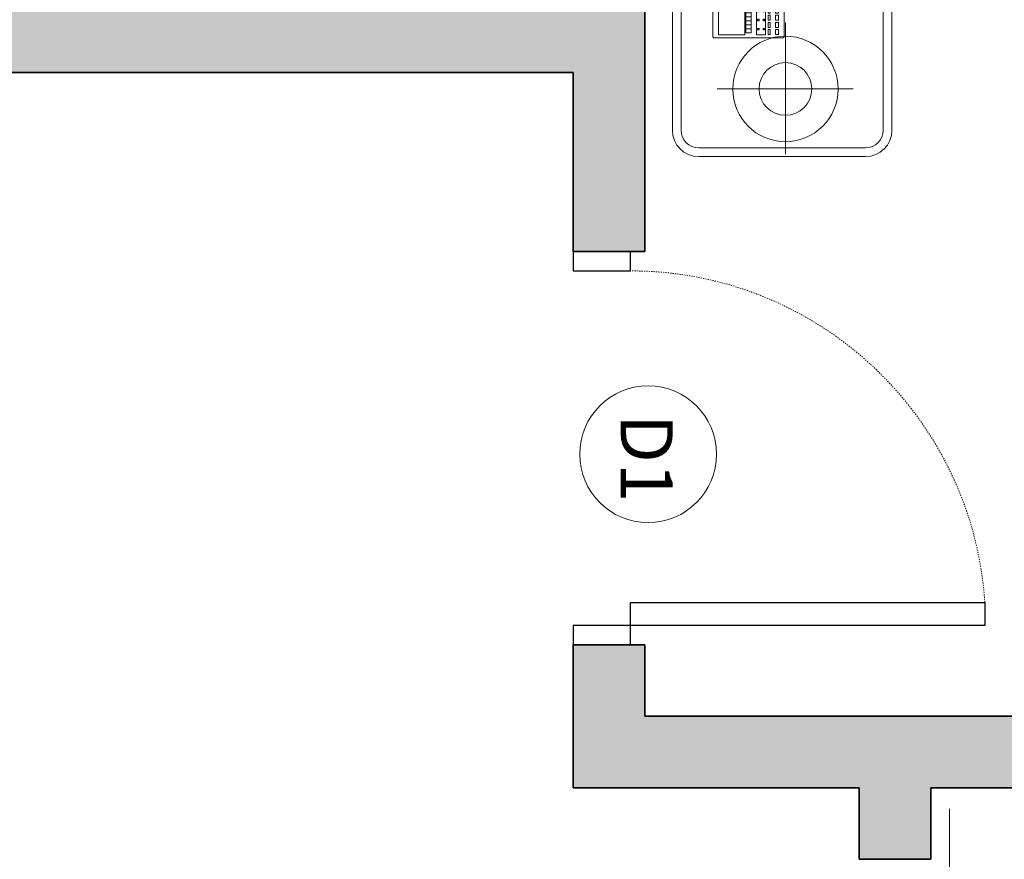
# Model space of a CAD drawing. Units: inches. Extents: x 2701 to 6846, y 811 to 2447.
# Tile 16 of 20: x 2926 to 3008, y 1300 to 1370. Entities that reach past the tile are written whole.
import ezdxf

# ---------------------------------------------------------------- set-up
doc = ezdxf.new("R2010")
doc.units = ezdxf.units.IN
doc.linetypes.add('HIDDEN4', pattern=[0.09375, 0.0625, -0.03125])
for name, color, linetype, lineweight in [('A-ANNO-IDEN', 7, 'Continuous', 13), ('A-DOOR', 4, 'Continuous', 25), ('A-DOOR-SWNG', 4, 'HIDDEN4', 13), ('A-FLOR-PATT', 252, 'Continuous', 13), ('A-FURN', 8, 'Continuous', 13), ('A-WALL', 7, 'Continuous', 35)]:
    doc.layers.add(name, color=color, linetype=linetype, lineweight=lineweight)
doc.layers.add('A-WALL-PATT', color=18, linetype='Continuous', lineweight=13, true_color=0x000000)
doc.styles.get("Standard").update_dxf_attribs({"font": 'arial.ttf'})

# ---------------------------------------------------------------- blocks, each defined once
blk = doc.blocks.new('A$C356F0359')
for p, q in [((0.5489, 2), (2.0492, 2)), ((0.5489, 1.9489), (0.5489, 2)), ((2.0492, 1.9489), (2.0492, 2)), ((0.4398, 1.9801), (0.0598, 1.9801)), ((2.5283, 1.9801), (2.1483, 1.9801)), ((0.4398, 1.9601), (0.0598, 1.9601)), ((2.5283, 1.9601), (2.1483, 1.9601)), ((2.0492, 1.9489), (0.5489, 1.9489)), ((1.998, 1.9289), (0.6001, 1.9289)), ((-0.0002, 1.9201), (-0.0002, 1.5401)), ((0.0198, 1.9201), (0.0198, 1.5401)), ((0.4798, 1.5401), (0.4798, 1.9201)), ((0.4998, 1.5401), (0.4998, 1.9201)), ((2.0883, 1.9201), (2.0883, 1.5401)), ((2.1083, 1.9201), (2.1083, 1.5401)), ((2.5683, 1.5401), (2.5683, 1.9201)), ((2.5883, 1.5401), (2.5883, 1.9201)), ((0.2725, 1.8879), (0.2702, 1.8856)), ((0.2702, 1.8856), (0.2702, 1.7279)), ((0.2725, 1.8879), (0.4531, 1.8879)), ((0.4016, 1.8787), (0.4062, 1.8845)), ((0.4062, 1.8845), (0.4405, 1.8845)), ((0.4405, 1.8845), (0.4462, 1.8787)), ((0.4531, 1.8879), (0.4553, 1.8856)), ((0.4553, 1.8856), (0.4553, 1.7279)), ((0.5489, 1.8977), (0.5489, 0.0512)), ((0.5689, 1.8977), (0.5689, 0.0512)), ((2.0292, 0.0512), (2.0292, 1.8977)), ((2.0492, 0.0512), (2.0492, 1.8977)), ((2.3306, 1.5822), (2.3306, 1.8917)), ((0.1539, 1.5681), (0.1539, 1.8777)), ((0.3913, 1.8753), (0.277, 1.8753)), ((0.277, 1.8753), (0.277, 1.8147)), ((0.3913, 1.8147), (0.3913, 1.8753)), ((0.4016, 1.7404), (0.4016, 1.8787)), ((0.4062, 1.881), (0.405, 1.8765)), ((0.405, 1.8765), (0.4153, 1.8662)), ((0.405, 1.8765), (0.405, 1.8456)), ((0.4108, 1.8833), (0.4062, 1.881)), ((0.4108, 1.8833), (0.4382, 1.8833)), ((0.4165, 1.8685), (0.4108, 1.8833)), ((0.4153, 1.8662), (0.4165, 1.8685)), ((0.4153, 1.8147), (0.4153, 1.8662)), ((0.4325, 1.8685), (0.4165, 1.8685)), ((0.4325, 1.8685), (0.4382, 1.8833)), ((0.4336, 1.8662), (0.4325, 1.8685)), ((0.4439, 1.8765), (0.4336, 1.8662)), ((0.4336, 1.8147), (0.4336, 1.8662)), ((0.4382, 1.8833), (0.4428, 1.881)), ((0.4428, 1.881), (0.4439, 1.8765)), ((0.4439, 1.8765), (0.4439, 1.8456)), ((0.4462, 1.8787), (0.4462, 1.7416)), ((0.405, 1.8456), (0.4073, 1.8399)), ((0.4073, 1.8399), (0.4108, 1.8342)), ((0.4416, 1.8399), (0.4382, 1.8342)), ((0.4439, 1.8456), (0.4416, 1.8399)), ((0.4108, 1.8342), (0.4119, 1.8262)), ((0.4119, 1.8262), (0.4119, 1.8147)), ((0.4382, 1.8342), (0.4371, 1.8262)), ((0.4371, 1.8262), (0.4371, 1.8147)), ((0.277, 1.8147), (0.3913, 1.8147)), ((0.3913, 1.8125), (0.2816, 1.8125)), ((0.2816, 1.8125), (0.2816, 1.801)), ((0.2816, 1.801), (0.3913, 1.801)), ((0.2907, 1.8125), (0.2907, 1.801)), ((0.2999, 1.8125), (0.2999, 1.801)), ((0.309, 1.8125), (0.309, 1.801)), ((0.3182, 1.8125), (0.3182, 1.801)), ((0.3273, 1.8125), (0.3273, 1.801)), ((0.3365, 1.8125), (0.3365, 1.801)), ((0.3913, 1.801), (0.3913, 1.8125)), ((0.4119, 1.793), (0.4119, 1.8147)), ((0.4153, 1.8147), (0.4153, 1.753)), ((0.4336, 1.8147), (0.4336, 1.753)), ((0.4371, 1.793), (0.4371, 1.8147)), ((0.277, 1.7885), (0.277, 1.7679)), ((0.3445, 1.7885), (0.277, 1.7885)), ((0.2885, 1.7862), (0.2885, 1.7827)), ((0.2919, 1.7862), (0.2885, 1.7862)), ((0.2885, 1.7827), (0.2919, 1.7827)), ((0.2919, 1.7736), (0.2885, 1.7736)), ((0.2885, 1.7736), (0.2885, 1.7702)), ((0.2919, 1.7827), (0.2919, 1.7862)), ((0.2919, 1.7702), (0.2919, 1.7736)), ((0.3125, 1.7862), (0.309, 1.7862)), ((0.309, 1.7862), (0.309, 1.7827)), ((0.309, 1.7827), (0.3125, 1.7827)), ((0.3125, 1.7736), (0.309, 1.7736)), ((0.309, 1.7736), (0.309, 1.7702)), ((0.3125, 1.7827), (0.3125, 1.7862)), ((0.3125, 1.7702), (0.3125, 1.7736)), ((0.333, 1.7862), (0.3296, 1.7862)), ((0.3296, 1.7862), (0.3296, 1.7827)), ((0.3296, 1.7827), (0.333, 1.7827)), ((0.333, 1.7736), (0.3296, 1.7736)), ((0.3296, 1.7736), (0.3296, 1.7702)), ((0.333, 1.7827), (0.333, 1.7862)), ((0.333, 1.7702), (0.333, 1.7736)), ((0.3445, 1.7679), (0.3445, 1.7885)), ((0.3548, 1.7759), (0.3548, 1.7827)), ((0.3548, 1.7827), (0.3639, 1.7827)), ((0.3639, 1.7759), (0.3548, 1.7759)), ((0.3639, 1.7827), (0.3639, 1.7759)), ((0.3685, 1.7827), (0.3776, 1.7827)), ((0.3685, 1.7759), (0.3685, 1.7827)), ((0.3776, 1.7759), (0.3685, 1.7759)), ((0.3776, 1.7827), (0.3776, 1.7759)), ((0.3822, 1.7759), (0.3822, 1.7827)), ((0.3822, 1.7827), (0.3913, 1.7827)), ((0.3913, 1.7759), (0.3822, 1.7759)), ((0.3913, 1.7827), (0.3913, 1.7759)), ((0.405, 1.7736), (0.4073, 1.7793)), ((0.405, 1.7427), (0.405, 1.7736)), ((0.4073, 1.7793), (0.4108, 1.785)), ((0.4108, 1.785), (0.4119, 1.793)), ((0.4382, 1.785), (0.4371, 1.793)), ((0.4416, 1.7793), (0.4382, 1.785)), ((0.4439, 1.7736), (0.4416, 1.7793)), ((0.4439, 1.7427), (0.4439, 1.7736)), ((0.277, 1.7679), (0.3445, 1.7679)), ((0.2782, 1.7622), (0.2782, 1.7576)), ((0.2896, 1.7622), (0.2782, 1.7622)), ((0.2782, 1.7576), (0.2896, 1.7576)), ((0.2885, 1.7702), (0.2919, 1.7702)), ((0.2896, 1.7576), (0.2896, 1.7622)), ((0.2942, 1.7622), (0.2942, 1.7576)), ((0.3056, 1.7622), (0.2942, 1.7622)), ((0.2942, 1.7576), (0.3056, 1.7576)), ((0.3056, 1.7576), (0.3056, 1.7622)), ((0.309, 1.7702), (0.3125, 1.7702)), ((0.3102, 1.7622), (0.3102, 1.7576)), ((0.3216, 1.7622), (0.3102, 1.7622)), ((0.3102, 1.7576), (0.3216, 1.7576)), ((0.3216, 1.7576), (0.3216, 1.7622)), ((0.3376, 1.7622), (0.3262, 1.7622)), ((0.3262, 1.7622), (0.3262, 1.7576)), ((0.3262, 1.7576), (0.3376, 1.7576)), ((0.3296, 1.7702), (0.333, 1.7702)), ((0.3376, 1.7576), (0.3376, 1.7622)), ((0.3548, 1.7633), (0.3548, 1.7702)), ((0.3548, 1.7702), (0.3639, 1.7702)), ((0.3639, 1.7633), (0.3548, 1.7633)), ((0.3548, 1.7564), (0.3639, 1.7564)), ((0.3548, 1.7496), (0.3548, 1.7564)), ((0.3639, 1.7496), (0.3548, 1.7496)), ((0.3639, 1.7702), (0.3639, 1.7633)), ((0.3639, 1.7564), (0.3639, 1.7496)), ((0.3685, 1.7633), (0.3685, 1.7702)), ((0.3685, 1.7702), (0.3776, 1.7702)), ((0.3776, 1.7633), (0.3685, 1.7633)), ((0.3685, 1.7564), (0.3776, 1.7564)), ((0.3685, 1.7496), (0.3685, 1.7564)), ((0.3776, 1.7496), (0.3685, 1.7496)), ((0.3776, 1.7702), (0.3776, 1.7633)), ((0.3776, 1.7564), (0.3776, 1.7496)), ((0.3822, 1.7633), (0.3822, 1.7702)), ((0.3822, 1.7702), (0.3913, 1.7702)), ((0.3913, 1.7633), (0.3822, 1.7633)), ((0.3822, 1.7576), (0.3913, 1.7576)), ((0.3822, 1.7507), (0.3822, 1.7576)), ((0.3913, 1.7507), (0.3822, 1.7507)), ((0.3913, 1.7702), (0.3913, 1.7633)), ((0.3913, 1.7576), (0.3913, 1.7507)), ((0.405, 1.7427), (0.4153, 1.753)), ((0.4165, 1.7507), (0.4108, 1.7359)), ((0.4153, 1.753), (0.4165, 1.7507)), ((0.4325, 1.7507), (0.4165, 1.7507)), ((0.4336, 1.753), (0.4325, 1.7507)), ((0.4325, 1.7507), (0.4382, 1.7359)), ((0.4439, 1.7427), (0.4336, 1.753)), ((0.2702, 1.7279), (0.2725, 1.7256)), ((0.2782, 1.745), (0.2896, 1.745)), ((0.2782, 1.7382), (0.2782, 1.745)), ((0.2896, 1.7382), (0.2782, 1.7382)), ((0.2896, 1.745), (0.2896, 1.7382)), ((0.2942, 1.745), (0.3056, 1.745)), ((0.2942, 1.7382), (0.2942, 1.745)), ((0.3056, 1.7382), (0.2942, 1.7382)), ((0.3056, 1.745), (0.3056, 1.7382)), ((0.3102, 1.745), (0.3216, 1.745)), ((0.3102, 1.7382), (0.3102, 1.745)), ((0.3216, 1.7382), (0.3102, 1.7382)), ((0.3216, 1.745), (0.3216, 1.7382)), ((0.3262, 1.7382), (0.3262, 1.745)), ((0.3262, 1.745), (0.3376, 1.745)), ((0.3376, 1.7382), (0.3262, 1.7382)), ((0.3376, 1.745), (0.3376, 1.7382)), ((0.3548, 1.737), (0.3548, 1.7439)), ((0.3548, 1.7439), (0.3639, 1.7439)), ((0.3639, 1.737), (0.3548, 1.737)), ((0.3639, 1.7439), (0.3639, 1.737)), ((0.3685, 1.737), (0.3685, 1.7439)), ((0.3685, 1.7439), (0.3776, 1.7439)), ((0.3776, 1.737), (0.3685, 1.737)), ((0.3776, 1.7439), (0.3776, 1.737)), ((0.3822, 1.7439), (0.3913, 1.7439)), ((0.3822, 1.737), (0.3822, 1.7439)), ((0.3913, 1.737), (0.3822, 1.737)), ((0.3913, 1.7439), (0.3913, 1.737)), ((0.4073, 1.7347), (0.4016, 1.7404)), ((0.4062, 1.7382), (0.405, 1.7427)), ((0.4108, 1.7359), (0.4062, 1.7382)), ((0.4234, 1.7347), (0.4073, 1.7347)), ((0.4108, 1.7359), (0.4234, 1.7359)), ((0.4233, 1.7393), (0.4235, 1.7294)), ((0.4268, 1.7393), (0.4233, 1.7393)), ((0.4235, 1.7294), (0.4263, 1.7179)), ((0.4274, 1.7301), (0.4268, 1.7393)), ((0.427, 1.7359), (0.4382, 1.7359)), ((0.4405, 1.7347), (0.4271, 1.7347)), ((0.429, 1.7227), (0.4274, 1.7301)), ((0.4382, 1.7359), (0.4428, 1.7382)), ((0.4462, 1.7416), (0.4405, 1.7347)), ((0.4428, 1.7382), (0.4439, 1.7427)), ((0.4553, 1.7279), (0.4531, 1.7256)), ((0.4622, 1.7459), (0.4553, 1.7484)), ((0.4553, 1.7439), (0.4604, 1.7425)), ((0.4604, 1.7425), (0.465, 1.7388)), ((0.4654, 1.7427), (0.4622, 1.7459)), ((0.465, 1.7388), (0.4662, 1.7372)), ((0.4678, 1.7405), (0.4654, 1.7427)), ((0.4662, 1.7372), (0.4686, 1.7374)), ((0.4686, 1.7374), (0.4662, 1.735)), ((0.4662, 1.735), (0.4755, 1.7268)), ((0.4721, 1.7421), (0.4678, 1.7405)), ((0.4741, 1.7401), (0.4721, 1.7421)), ((0.4725, 1.7366), (0.4741, 1.7401)), ((0.4753, 1.7388), (0.4725, 1.7366)), ((0.4783, 1.7356), (0.4753, 1.7388)), ((0.4755, 1.7268), (0.4906, 1.7139)), ((0.4759, 1.729), (0.4783, 1.7356)), ((0.4821, 1.7322), (0.4759, 1.729)), ((0.4874, 1.7272), (0.4821, 1.7322)), ((0.4862, 1.7199), (0.4874, 1.7272)), ((2.4819, 1.7366), (2.1818, 1.7366)), ((0.3052, 1.7226), (0.0051, 1.7226)), ((0.4244, 1.7256), (0.2725, 1.7256)), ((0.4263, 1.7179), (0.429, 1.707)), ((0.4531, 1.7256), (0.4284, 1.7256)), ((0.429, 1.707), (0.4288, 1.701)), ((0.4318, 1.7119), (0.429, 1.7227)), ((0.4325, 1.7063), (0.4318, 1.7119)), ((0.4323, 1.7003), (0.4325, 1.7063)), ((0.4914, 1.7231), (0.4862, 1.7199)), ((0.4908, 1.7135), (0.4984, 1.6917)), ((0.4958, 1.7185), (0.4914, 1.7231)), ((0.494, 1.7135), (0.4958, 1.7185)), ((0.501, 1.7142), (0.494, 1.7135)), ((0.4964, 1.7047), (0.5031, 1.7072)), ((0.5038, 1.7049), (0.4964, 1.7047)), ((0.5031, 1.7072), (0.501, 1.7142)), ((0.5054, 1.6996), (0.5038, 1.7049)), ((0.427, 1.697), (0.4265, 1.6915)), ((0.4265, 1.6915), (0.4332, 1.6903)), ((0.4332, 1.6903), (0.4267, 1.6864)), ((0.4267, 1.6864), (0.4272, 1.6801)), ((0.4295, 1.6996), (0.427, 1.697)), ((0.4288, 1.701), (0.4295, 1.6996)), ((0.4364, 1.6973), (0.4323, 1.7003)), ((0.4355, 1.6919), (0.4364, 1.6973)), ((0.4367, 1.6774), (0.4355, 1.6919)), ((0.4984, 1.6917), (0.4952, 1.6744)), ((0.5005, 1.695), (0.5054, 1.6996)), ((0.5068, 1.695), (0.5005, 1.695)), ((0.5008, 1.6871), (0.5079, 1.6892)), ((0.5068, 1.6836), (0.5008, 1.6871)), ((0.5058, 1.679), (0.5068, 1.6836)), ((0.5079, 1.6892), (0.5068, 1.695)), ((0.4272, 1.6801), (0.4346, 1.6794)), ((0.4346, 1.6794), (0.4281, 1.6744)), ((0.4281, 1.6744), (0.4311, 1.669)), ((0.4311, 1.669), (0.4381, 1.6704)), ((0.4381, 1.6704), (0.4348, 1.6639)), ((0.4348, 1.6639), (0.4383, 1.6598)), ((0.4455, 1.6663), (0.4367, 1.6774)), ((0.4383, 1.6598), (0.4436, 1.6637)), ((0.4436, 1.6637), (0.4427, 1.6575)), ((0.4577, 1.6598), (0.4455, 1.6663)), ((0.4471, 1.6547), (0.4526, 1.6593)), ((0.4526, 1.6593), (0.4519, 1.6517)), ((0.4716, 1.6586), (0.4577, 1.6598)), ((0.485, 1.6644), (0.4716, 1.6586)), ((0.4843, 1.6538), (0.4836, 1.6607)), ((0.4836, 1.6607), (0.4885, 1.6547)), ((0.4952, 1.6744), (0.485, 1.6644)), ((0.4922, 1.6579), (0.4894, 1.6642)), ((0.4894, 1.6642), (0.4959, 1.6614)), ((0.4957, 1.6704), (0.5024, 1.6683)), ((0.4989, 1.6642), (0.4957, 1.6704)), ((0.4959, 1.6614), (0.4989, 1.6642)), ((0.5042, 1.673), (0.4987, 1.6792)), ((0.4987, 1.6792), (0.5058, 1.679)), ((0.5024, 1.6683), (0.5042, 1.673)), ((0.4427, 1.6575), (0.4471, 1.6547)), ((0.4519, 1.6517), (0.4568, 1.6503)), ((0.4568, 1.6503), (0.4598, 1.6565)), ((0.4598, 1.6565), (0.4626, 1.6503)), ((0.4626, 1.6503), (0.4665, 1.6498)), ((0.4665, 1.6498), (0.4681, 1.6565)), ((0.4681, 1.6565), (0.4707, 1.6491)), ((0.4707, 1.6491), (0.4751, 1.6503)), ((0.4751, 1.6503), (0.4753, 1.6565)), ((0.4753, 1.6565), (0.4806, 1.6519)), ((0.4806, 1.6519), (0.4843, 1.6538)), ((0.4885, 1.6547), (0.4922, 1.6579)), ((0.0598, 1.5001), (0.4398, 1.5001)), ((0.0598, 1.4801), (0.4398, 1.4801)), ((2.1483, 1.5001), (2.5283, 1.5001)), ((2.1483, 1.4801), (2.5283, 1.4801)), ((0.6001, 0.02), (1.998, 0.02)), ((0.6001, 0), (1.998, 0))]:
    blk.add_line(p, q)
at = {"linetype": 'ByBlock'}
for p, q in [((0.6001, 1.9147), (1.282, 1.9147)), ((0.6001, 1.6759), (0.6001, 1.9147)), ((1.282, 1.9147), (1.282, 1.6759)), ((1.3161, 1.9147), (1.998, 1.9147)), ((1.3161, 1.6759), (1.3161, 1.9147)), ((1.998, 1.9147), (1.998, 1.6759)), ((1.282, 1.6759), (0.6001, 1.6759)), ((1.998, 1.6759), (1.3161, 1.6759)), ((1.0687, 1.6418), (0.5489, 1.6418)), ((1.4185, 1.5053), (0.5489, 1.5053))]:
    blk.add_line(p, q, dxfattribs=at)
for centre in [(0.1539, 1.7226), (2.3306, 1.7366)]:
    blk.add_circle(centre, 0.12, dxfattribs=at)
for centre in [(2.3306, 1.7366), (0.1539, 1.7226)]:
    blk.add_circle(centre, 0.06)
for centre, radius, start, end in [((0.0598, 1.9201), 0.06, 90, 180), ((0.4398, 1.9201), 0.06, 0, 90), ((2.1483, 1.9201), 0.06, 90, 180), ((2.5283, 1.9201), 0.06, 0, 90), ((0.0598, 1.9201), 0.04, 90, 180), ((0.4398, 1.9201), 0.04, 0, 90), ((2.1483, 1.9201), 0.04, 90, 180), ((2.5283, 1.9201), 0.04, 0, 90), ((0.6001, 1.8977), 0.0512, 90, 180), ((0.6001, 1.8977), 0.0312, 90, 180), ((1.998, 1.8977), 0.0512, 0, 90), ((1.998, 1.8977), 0.0312, 0, 90), ((0.0598, 1.5401), 0.06, 180, 270), ((0.0598, 1.5401), 0.04, 180, 270), ((0.4398, 1.5401), 0.04, 270, 0), ((0.4398, 1.5401), 0.06, 270, 0), ((2.1483, 1.5401), 0.06, 180, 270), ((2.1483, 1.5401), 0.04, 180, 270), ((2.5283, 1.5401), 0.06, 270, 0), ((2.5283, 1.5401), 0.04, 270, 0), ((1.1471, 0.7332), 0.3575, 102.4782, 140.4625), ((1.9086, 1.3124), 0.8697, 195.336, 226.4193), ((0.3249, 0.4335), 0.9879, 28.4971, 41.0566), ((0.9965, 0.4273), 0.548, 103.2034, 117.0362), ((1.6529, 1.7059), 1.0798, 223.6306, 251.4288), ((0.4451, 0.4375), 0.5655, 5.3391, 57.6895), ((0.4517, 0.5274), 0.4879, 10.6986, 52.6864), ((1.8195, 1.3719), 1.1652, 203.0642, 220.3209), ((0.5617, 0.4344), 0.7874, 18.3527, 36.6851), ((-0.021, 2.4319), 2.1977, 305.2966, 307.2418), ((1.4135, 0.487), 0.3575, 154.0418, 192.0262), ((1.1372, -0.3434), 0.9879, 80.0607, 92.6202), ((1.2836, -0.1573), 0.7874, 69.9163, 88.2487), ((1.5949, 0.9312), 0.734, 205.259, 216.9351), ((1.3641, 0.0041), 0.6085, 71.81, 120.1351), ((1.44, 0.1186), 0.4774, 76.1849, 142.0017), ((-0.6432, 0.628), 2.1977, 349.4884, 358.8054), ((-0.021, 2.4319), 2.1977, 297.9248, 299.3793), ((1.5595, 0.1789), 0.548, 154.767, 168.5998), ((1.2647, 0.9578), 0.6885, 250.2936, 293.6414), ((1.3312, 1.4107), 1.1652, 254.6278, 271.8845), ((1.5368, 0.9609), 0.734, 256.8226, 268.4988), ((0.5943, 0.0454), 0.0458, 172.7599, 277.2401), ((0.5943, 0.0454), 0.0258, 172.7599, 277.2401), ((2.0038, 0.0454), 0.0458, 262.7599, 7.2401), ((2.0038, 0.0454), 0.0258, 262.7599, 7.2401)]:
    blk.add_arc(centre, radius, start, end)
for centre, radius, start, end in [((0.1906, 1.7953), 0.4265, 343.7398, 16.2602), ((1.6914, 1.7953), 0.4265, 163.7398, 196.2602), ((0.9067, 1.7953), 0.4265, 343.7398, 16.2602), ((2.4075, 1.7953), 0.4265, 163.7398, 196.2602), ((0.9303, 0.657), 0.9853, 61.4328, 88.1261), ((1.0826, 0.5712), 1.0706, 72.1966, 90.7418), ((2.1368, 4.5996), 3.0955, 256.4201, 268.3789), ((2.0056, 2.7745), 1.3903, 244.2427, 271.7984)]:
    blk.add_arc(centre, radius, start, end, dxfattribs=at)
blk = doc.blocks.new('DOOR-D1-33IN-PANEL-FRAME')
blk.add_lwpolyline([(0, 33), (0, 31.373), (4.798, 31.373), (4.798, 33), (0, 33)], close=True)
for points in [[(4.318, 33), (0.48, 33)], [(4.798, 0), (4.798, 3.546), (34.543, 3.546), (34.543, 1.627), (0, 1.627), (0, 0)], [(0, 0), (4.798, 0)], [(4.318, 0), (0.48, 0)]]:
    blk.add_lwpolyline(points)

msp = doc.modelspace()

# ---------------------------------------------------------------- hatches: boundary and pattern name
at = {"layer": 'A-FLOR-PATT'}
h = msp.add_hatch(dxfattribs=at)
h.set_pattern_fill('ANGLE', color=256)
h.set_pattern_definition([(0, (0, 0), (0, 6.985), [5.08, -1.905]), (90, (0, 0), (-6.985, 4e-16), [5.08, -1.905])])
h.paths.add_polyline_path([(2841.813, 1296.511, -0.109453), (2842.614, 1300.129, -0.102375), (2844.977, 1303.302, -0.093743), (2848.426, 1305.368, -0.062463), (2851.367, 1306.05), (2785.971, 1306.05), (2785.971, 1258.05), (2827.971, 1258.05), (2827.971, 1256.412), (2829.451, 1256.412, -0.394827), (2854.747, 1283.453), (2856.492, 1283.453), (2856.492, 1256.412), (2857.971, 1256.412), (2857.971, 1258.05), (2863.971, 1258.05), (2863.971, 1306.05), (2853.867, 1306.05, -0.062463), (2856.808, 1305.368, -0.093743), (2860.257, 1303.302, -0.102375), (2862.62, 1300.129, -0.109453), (2863.421, 1296.511, -0.109453), (2862.62, 1292.893, -0.102375), (2860.257, 1289.72, -0.093738), (2856.808, 1287.654, -0.088425), (2852.617, 1286.907, -0.088425), (2848.426, 1287.654, -0.093738), (2844.977, 1289.72, -0.102375), (2842.614, 1292.893, -0.109453)])
h.paths.add_polyline_path([(2805.215, 1273.877, -0.141745), (2808.319, 1271.773, -0.184983), (2809.774, 1267.974, -0.184983), (2808.319, 1264.176, -0.141745), (2805.215, 1262.071, -0.152244), (2799.994, 1261.796, -0.025614), (2799.369, 1261.945), (2794.365, 1263.418), (2794.365, 1263.405, -0.111242), (2793.993, 1261.915, -0.033889), (2793.114, 1260.114, -0.286745), (2792.376, 1259.652), (2787.581, 1259.652, -0.414214), (2787.153, 1260.08), (2787.153, 1267.974), (2787.153, 1275.869, -0.414214), (2787.581, 1276.297), (2792.376, 1276.297, -0.286745), (2793.114, 1275.835, -0.033889), (2793.993, 1274.033, -0.105104), (2794.362, 1272.628), (2794.365, 1272.53), (2799.369, 1274.003, -0.025614), (2799.994, 1274.153, -0.152244)], flags=16)
h.paths.add_polyline_path([(2804.681, 1272.34, -0.144945), (2807.088, 1270.709, -0.0358), (2807.447, 1270.253, -0.133285), (2807.893, 1268.608), (2807.893, 1267.974), (2807.893, 1267.341, -0.133285), (2807.447, 1265.696, -0.0358), (2807.088, 1265.24, -0.144945), (2804.681, 1263.609, -0.155404), (2800.343, 1263.386, -0.364511), (2796.485, 1267.974, -0.364511), (2800.343, 1272.563, -0.155404)], flags=0)
h.paths.add_polyline_path([(2800.016, 1268.901, 0.169298), (2799.131, 1268.116, 0.076667), (2799.1, 1267.974, 0.076667), (2799.131, 1267.833, 0.169298), (2800.016, 1267.047, 0.305219), (2800.365, 1267.156, 0.169535), (2800.651, 1267.974, 0.169535), (2800.365, 1268.792, 0.305219)], flags=0)
h.paths.add_polyline_path([(2971.971, 1456.05), (2923.971, 1456.05), (2923.971, 1408.05), (2922.333, 1408.05), (2922.333, 1406.571, -0.394827), (2949.374, 1381.274), (2949.374, 1379.529), (2922.333, 1379.529), (2922.333, 1378.05), (2923.971, 1378.05), (2923.971, 1372.05), (2971.971, 1372.05)])
h.paths.add_polyline_path([(2939.818, 1436.526, -0.141745), (2937.713, 1433.423, -0.184983), (2933.915, 1431.968, -0.184983), (2930.117, 1433.423, -0.141745), (2928.012, 1436.526, -0.152244), (2927.736, 1441.747, -0.025614), (2927.886, 1442.373), (2929.359, 1447.376), (2929.346, 1447.377, -0.111242), (2927.856, 1447.748, -0.033889), (2926.054, 1448.627, -0.286745), (2925.593, 1449.366), (2925.593, 1454.16, -0.414214), (2926.021, 1454.589), (2933.915, 1454.589), (2941.809, 1454.589, -0.414207), (2942.237, 1454.16), (2942.237, 1449.366, -0.286745), (2941.776, 1448.627, -0.033889), (2939.974, 1447.748, -0.105104), (2938.569, 1447.38), (2938.471, 1447.376), (2939.944, 1442.373, -0.025614), (2940.094, 1441.747, -0.152244)], flags=16)
h.paths.add_polyline_path([(2938.281, 1437.06, -0.144945), (2936.649, 1434.654, -0.0358), (2936.193, 1434.294, -0.133285), (2934.548, 1433.848), (2933.915, 1433.848), (2933.281, 1433.848, -0.133285), (2931.636, 1434.294, -0.0358), (2931.181, 1434.654, -0.144945), (2929.549, 1437.06, -0.155404), (2929.326, 1441.398, -0.364511), (2933.915, 1445.256, -0.364511), (2938.503, 1441.398, -0.155404)], flags=0)
h.paths.add_polyline_path([(2969.158, 1392.045, -0.093743), (2971.224, 1388.596, -0.088421), (2971.971, 1384.405, -0.088421), (2971.224, 1380.214, -0.093743), (2969.158, 1376.765, -0.102375), (2965.986, 1374.402, -0.109453), (2962.367, 1373.6, -0.109453), (2958.749, 1374.402, -0.102375), (2955.576, 1376.765, -0.093738), (2953.511, 1380.213, -0.088425), (2952.764, 1384.405, -0.088425), (2953.511, 1388.596, -0.093738), (2955.576, 1392.045, -0.102375), (2958.749, 1394.407, -0.109453), (2962.367, 1395.209, -0.109453), (2965.986, 1394.407, -0.102375)], flags=0)
edge = h.paths.add_edge_path(flags=16)
edge.add_arc((2961.075, 1384.859), 10.199, 20.2132, 41.63359, ccw=False)
edge.add_spline(control_points=[(2970.646, 1388.383), (2970.459, 1387.83), (2970.004, 1386.481), (2971.435, 1384.396), (2969.868, 1382.339), (2970.408, 1381.011), (2970.646, 1380.426)], knot_values=[0, 0, 0, 0, 0.041109, 0.100337, 0.155913, 0.199586, 0.199586, 0.199586, 0.199586], degree=3, periodic=0)
edge.add_arc((2961.075, 1383.95), 10.199, 318.36641, 339.7868, ccw=False)
edge.add_arc((2961.862, 1383.25), 9.145, 294.98529, 318.36641, ccw=False)
edge.add_arc((2962.367, 1382.166), 7.949, 269.99999, 294.98535, ccw=False)
edge.add_arc((2962.367, 1382.166), 7.949, 245.01465, 270.00002, ccw=False)
edge.add_arc((2962.873, 1383.25), 9.145, 221.63359, 245.01471, ccw=False)
edge.add_arc((2963.66, 1383.95), 10.199, 200.21296, 221.63359, ccw=False)
edge.add_arc((2964.894, 1384.405), 11.514, 180, 200.21296, ccw=False)
edge.add_arc((2964.894, 1384.405), 11.514, 159.78704, 179.99999, ccw=False)
edge.add_arc((2963.66, 1384.859), 10.199, 138.36641, 159.78704, ccw=False)
edge.add_arc((2962.873, 1385.559), 9.145, 114.98529, 138.36641, ccw=False)
edge.add_arc((2962.367, 1386.643), 7.949, 89.99999, 114.98534, ccw=False)
edge.add_arc((2962.367, 1386.643), 7.949, 65.01465, 90.00002, ccw=False)
edge.add_arc((2961.862, 1385.559), 9.145, 41.63359, 65.01471, ccw=False)
h.paths.add_polyline_path([(2963.81, 1393.327, -0.126458), (2966.613, 1390.683, -0.141697), (2967.169, 1388.761), (2967.169, 1387.406, -1), (2969.57, 1387.406, -0.414214), (2968.37, 1386.205), (2963.568, 1385.005, 0.146218), (2963.311, 1384.663), (2968.97, 1385.64), (2968.97, 1383.155), (2963.317, 1384.13, 0.140312), (2963.568, 1383.804), (2968.37, 1382.604, -0.414214), (2969.57, 1381.403, -1), (2967.169, 1381.403), (2967.169, 1380.04, -0.149025), (2966.557, 1378.032, -0.012759), (2966.265, 1377.619, -0.106303), (2963.81, 1375.482, -0.126822), (2961.167, 1374.801, -0.126822), (2958.524, 1375.482, -0.106303), (2956.069, 1377.619, -0.085722), (2954.537, 1380.623, -0.075351), (2953.964, 1384.405, -0.075351), (2954.537, 1388.187, -0.085722), (2956.069, 1391.19, -0.106303), (2958.524, 1393.327, -0.126822), (2961.167, 1394.009, -0.126822)], flags=0)
h.paths.add_polyline_path([(2934.842, 1441.725, 0.169298), (2934.056, 1442.61, 0.076667), (2933.915, 1442.641, 0.076667), (2933.773, 1442.61, 0.169298), (2932.988, 1441.725, 0.305219), (2933.097, 1441.376, 0.169535), (2933.915, 1441.09, 0.169535), (2934.733, 1441.376, 0.305219)], flags=0)
h.paths.add_polyline_path([(2969.324, 1387.406, -1), (2967.416, 1387.406, -1)], flags=0)
h.paths.add_polyline_path([(2968.831, 1387.406, -1), (2967.909, 1387.406, -1)], flags=0)
h.paths.add_polyline_path([(2962.13, 1384.357, -1), (2960.209, 1384.357, -1)], flags=0)
h.paths.add_polyline_path([(2961.801, 1384.357, -1), (2960.538, 1384.357, -1)], flags=0)
h.paths.add_polyline_path([(2969.324, 1381.403, -1), (2967.416, 1381.403, -1)], flags=0)
h.paths.add_polyline_path([(2968.831, 1381.403, -1), (2967.909, 1381.403, -1)], flags=0)
h.paths.add_polyline_path([(3085.971, 1306.05), (3001.971, 1306.05), (3001.971, 1300.05), (3000.333, 1300.05), (3000.333, 1298.571), (3027.374, 1298.571), (3027.374, 1296.826, -0.394827), (3000.333, 1271.529), (3000.333, 1270.05), (3001.971, 1270.05), (3001.971, 1258.05), (3085.971, 1258.05)])
h.paths.add_polyline_path([(3033.333, 1274.445, -0.102375), (3035.696, 1271.272, -0.109453), (3036.497, 1267.654, -0.109453), (3035.696, 1264.036, -0.102375), (3033.333, 1260.863, -0.093743), (3029.884, 1258.797, -0.088421), (3025.693, 1258.05, -0.088421), (3021.502, 1258.797, -0.093743), (3018.053, 1260.863, -0.102375), (3015.69, 1264.036, -0.109453), (3014.888, 1267.654, -0.109453), (3015.69, 1271.272, -0.102375), (3018.053, 1274.445, -0.093738), (3021.502, 1276.511, -0.088425), (3025.693, 1277.258, -0.088425), (3029.884, 1276.511, -0.093738)], flags=0)
edge = h.paths.add_edge_path(flags=16)
edge.add_arc((3026.847, 1267.149), 9.145, 24.98529, 48.36641, ccw=False)
edge.add_arc((3027.931, 1267.654), 7.949, -0.00001, 24.98534, ccw=False)
edge.add_arc((3027.931, 1267.654), 7.949, -24.98534, 0.00002, ccw=False)
edge.add_arc((3026.847, 1268.159), 9.145, 311.63359, 335.01471, ccw=False)
edge.add_arc((3026.147, 1268.947), 10.199, 290.2132, 311.63359, ccw=False)
edge.add_spline(control_points=[(3029.671, 1259.376), (3029.087, 1259.613), (3027.759, 1260.153), (3025.702, 1258.586), (3023.617, 1260.017), (3022.267, 1259.562), (3021.715, 1259.376)], knot_values=[0, 0, 0, 0, 0.043673, 0.099248, 0.158477, 0.199586, 0.199586, 0.199586, 0.199586], degree=3, periodic=0)
edge.add_arc((3025.239, 1268.947), 10.199, 228.36641, 249.7868, ccw=False)
edge.add_arc((3024.538, 1268.159), 9.145, 204.98529, 228.36641, ccw=False)
edge.add_arc((3023.454, 1267.654), 7.949, 179.99999, 204.98534, ccw=False)
edge.add_arc((3023.454, 1267.654), 7.949, 155.01465, 180.00002, ccw=False)
edge.add_arc((3024.538, 1267.149), 9.145, 131.63359, 155.01471, ccw=False)
edge.add_arc((3025.239, 1266.361), 10.199, 110.21296, 131.63359, ccw=False)
edge.add_arc((3025.693, 1265.127), 11.514, 90, 110.21296, ccw=False)
edge.add_arc((3025.693, 1265.127), 11.514, 69.78704, 89.99999, ccw=False)
edge.add_arc((3026.147, 1266.361), 10.199, 48.36641, 69.78704, ccw=False)
h.paths.add_polyline_path([(3032.478, 1273.952, -0.106303), (3034.615, 1271.497, -0.126822), (3035.297, 1268.854, -0.126822), (3034.615, 1266.212, -0.106303), (3032.478, 1263.757, -0.012759), (3032.066, 1263.464, -0.149025), (3030.057, 1262.852), (3028.694, 1262.852, -0.414214), (3029.895, 1261.652, -1), (3027.494, 1261.652), (3026.293, 1266.453, 0.140312), (3025.968, 1266.704), (3026.943, 1261.051), (3024.458, 1261.051), (3025.434, 1266.71, 0.146218), (3025.093, 1266.453), (3023.892, 1261.652, -1), (3021.491, 1261.652, -0.414214), (3022.692, 1262.852), (3021.337, 1262.852, -0.141697), (3019.415, 1263.408, -0.126458), (3016.77, 1266.212, -0.126822), (3016.089, 1268.854, -0.126822), (3016.77, 1271.497, -0.106303), (3018.908, 1273.952, -0.085722), (3021.911, 1275.484, -0.075351), (3025.693, 1276.057, -0.075351), (3029.475, 1275.484, -0.085722)], flags=0)
h.paths.add_polyline_path([(3072.365, 1280.002, -0.184983), (3076.163, 1281.457, -0.184983), (3079.961, 1280.002, -0.141745), (3082.066, 1276.898, -0.152244), (3082.342, 1271.678, -0.025614), (3082.192, 1271.052), (3080.719, 1266.048), (3080.817, 1266.045, -0.105104), (3082.222, 1265.676, -0.033889), (3084.024, 1264.798, -0.286745), (3084.485, 1264.059), (3084.485, 1259.264, -0.41422), (3084.057, 1258.836), (3076.163, 1258.836), (3068.269, 1258.836, -0.414214), (3067.841, 1259.264), (3067.841, 1264.059, -0.286745), (3068.302, 1264.798, -0.033889), (3070.104, 1265.676, -0.105104), (3071.509, 1266.045), (3071.607, 1266.048), (3070.134, 1271.052, -0.025614), (3069.984, 1271.678, -0.152244), (3070.26, 1276.898, -0.141745)], flags=16)
h.paths.add_polyline_path([(3073.429, 1278.771, -0.0358), (3073.885, 1279.13, -0.133285), (3075.529, 1279.577), (3076.163, 1279.577), (3076.797, 1279.577, -0.133285), (3078.441, 1279.13, -0.0358), (3078.897, 1278.771, -0.144945), (3080.529, 1276.364, -0.155404), (3080.752, 1272.026, -0.364511), (3076.163, 1268.168, -0.364511), (3071.574, 1272.026, -0.155404), (3071.797, 1276.364, -0.144945)], flags=0)
h.paths.add_polyline_path([(3026.7, 1268.852, -1), (3024.78, 1268.852, -1)], flags=0)
h.paths.add_polyline_path([(3026.372, 1268.852, -1), (3025.108, 1268.852, -1)], flags=0)
h.paths.add_polyline_path([(3075.269, 1271.624, 0.157677), (3076.022, 1270.814, 0.076667), (3076.163, 1270.783, 0.076667), (3076.304, 1270.814, 0.157677), (3077.058, 1271.624, 0.374626), (3076.981, 1272.048, 0.169535), (3076.163, 1272.334, 0.169535), (3075.345, 1272.048, 0.374626)], flags=0)
h.paths.add_polyline_path([(3029.648, 1261.652, -1), (3027.74, 1261.652, -1)], flags=0)
h.paths.add_polyline_path([(3029.155, 1261.652, -1), (3028.233, 1261.652, -1)], flags=0)
h.paths.add_polyline_path([(3023.646, 1261.652, -1), (3021.738, 1261.652, -1)], flags=0)
h.paths.add_polyline_path([(3023.152, 1261.652, -1), (3022.231, 1261.652, -1)], flags=0)
h.paths.add_polyline_path([(2810.573, 1281.222), (2833.311, 1281.222), (2833.311, 1296.429), (2810.573, 1296.429)], flags=24)
h.paths.add_polyline_path([(2937.545, 1410.244), (2960.208, 1410.244), (2960.208, 1425.452), (2937.545, 1425.452)], flags=24)
h.paths.add_polyline_path([(3043.228, 1273.099), (3065.891, 1273.099), (3065.891, 1288.306), (3043.228, 1288.306)], flags=24)
at = {"layer": 'A-WALL-PATT'}
h = msp.add_hatch(color=256, dxfattribs=at)
h.dxf.hatch_style = 1
h.paths.add_polyline_path([(3085.971, 1456.05), (3085.971, 1348.05), (3091.971, 1348.05), (3091.971, 1360.05), (3091.971, 1462.05), (2960.086, 1462.05), (2960.086, 1456.05), (2971.971, 1456.05), (2971.971, 1372.05), (2923.971, 1372.05), (2923.971, 1378.05), (2917.971, 1378.05), (2917.971, 1351.05), (2923.971, 1351.05), (2923.971, 1366.05), (2971.971, 1366.05), (2971.971, 1351.05), (2976.769, 1351.05), (2977.971, 1351.05), (2977.971, 1456.05)])
h.paths.add_polyline_path([(2779.971, 1462.05), (2779.971, 1342.05), (2785.971, 1342.05), (2785.971, 1456.05), (2917.971, 1456.05), (2917.971, 1408.05), (2922.333, 1408.05), (2923.971, 1408.05), (2923.971, 1456.05), (2937.086, 1456.05), (2937.086, 1462.05)])
h.paths.add_polyline_path([(2779.971, 1306.05), (2779.971, 1294.241), (2785.971, 1294.241), (2785.971, 1306.05), (2851.367, 1306.05, -0.025815), (2852.617, 1306.115, -0.025815), (2853.867, 1306.05), (2863.971, 1306.05), (2863.971, 1258.05), (2857.971, 1258.05), (2857.971, 1252.05), (2878.971, 1252.05), (2878.971, 1258.05), (2869.971, 1258.05), (2869.971, 1306.05), (2923.971, 1306.05), (2923.971, 1318.05), (2919.174, 1318.05), (2917.971, 1318.05), (2917.971, 1312.05), (2785.971, 1312.05), (2785.971, 1318.05), (2779.971, 1318.05)])
h.paths.add_polyline_path([(2785.971, 1252.05), (2827.971, 1252.05), (2827.971, 1256.412), (2827.971, 1258.05), (2785.971, 1258.05), (2785.971, 1271.241), (2779.971, 1271.241), (2779.971, 1174.05), (2785.971, 1174.05)])
h.paths.add_polyline_path([(2779.971, 1030.05), (2869.971, 1030.05), (2869.971, 1036.05), (2785.971, 1036.05), (2785.971, 1126.05), (2917.971, 1126.05), (2917.971, 1120.05), (2923.971, 1120.05), (2923.971, 1258.05), (2911.971, 1258.05), (2911.971, 1253.252), (2911.971, 1252.05), (2917.971, 1252.05), (2917.971, 1132.05), (2785.971, 1132.05), (2785.971, 1144.05), (2779.971, 1144.05)])
h.paths.add_polyline_path([(2935.971, 1030.05), (2935.971, 1033.05), (2935.971, 1036.05), (2923.971, 1036.05), (2923.971, 1087.05), (2919.174, 1087.05), (2917.971, 1087.05), (2917.971, 1036.05), (2893.971, 1036.05), (2893.971, 1030.05)])
h.paths.add_polyline_path([(2971.971, 1036.05), (2971.971, 1030.05), (3091.971, 1030.05), (3091.971, 1060.05), (3085.971, 1060.05), (3085.971, 1036.05)])
h.paths.add_polyline_path([(3085.971, 1084.05), (3091.971, 1084.05), (3091.971, 1096.05), (3091.971, 1268.891), (3085.971, 1268.891), (3085.971, 1258.05), (3001.971, 1258.05), (3001.971, 1270.05), (2995.971, 1270.05), (2995.971, 1252.05), (3085.971, 1252.05)])
h.paths.add_polyline_path([(3085.971, 1306.05), (3085.971, 1291.891), (3091.971, 1291.891), (3091.971, 1318.05), (3085.971, 1318.05), (3085.971, 1312.05), (2977.971, 1312.05), (2977.971, 1318.05), (2971.971, 1318.05), (2971.971, 1306.05), (2995.971, 1306.05), (2995.971, 1300.05), (3000.333, 1300.05), (3001.971, 1300.05), (3001.971, 1306.05)])

# ---------------------------------------------------------------- linework, layer by layer
at = {"layer": 'A-ANNO-IDEN'}
msp.add_circle((2978.253, 1334.036), 5.739, dxfattribs=at)
at = {"layer": 'A-DOOR-SWNG'}
msp.add_arc((2976.769, 1319.611), 29.812, 3.8183, 90, dxfattribs=at)
at = {"layer": 'A-WALL'}
for p, q in [((2977.971, 1351.05), (2977.971, 1456.05)), ((2971.971, 1366.05), (2923.971, 1366.05)), ((2971.971, 1351.05), (2971.971, 1366.05)), ((2977.971, 1351.05), (2971.971, 1351.05)), ((2971.971, 1306.05), (2971.971, 1318.05)), ((2977.971, 1318.05), (2971.971, 1318.05)), ((2977.971, 1312.05), (2977.971, 1318.05)), ((3085.971, 1312.05), (2977.971, 1312.05)), ((2995.971, 1306.05), (2971.971, 1306.05)), ((2995.971, 1306.05), (2995.971, 1300.05)), ((3085.971, 1306.05), (3001.971, 1306.05)), ((3001.971, 1306.05), (3001.971, 1300.05)), ((3001.971, 1300.05), (2995.971, 1300.05))]:
    msp.add_line(p, q, dxfattribs=at)

# ---------------------------------------------------------------- block references
at = {"layer": 'A-DOOR'}
msp.add_blockref('DOOR-D1-33IN-PANEL-FRAME', (2971.971, 1318.05), dxfattribs=at)
at = {"layer": 'A-FURN', "xscale": 36.85134703248138, "yscale": 36.85134703248138, "zscale": 36.85134703248138, "rotation": 90}
msp.add_blockref('A$C356F0359', (3053.257, 1359.007), dxfattribs=at)

# ---------------------------------------------------------------- texts
at = {"layer": 'A-ANNO-IDEN', "insert": (2980.317, 1337.405), "char_height": 4.3649, "attachment_point": 1, "rotation": 270}
msp.add_mtext('D1', dxfattribs=at)

doc.saveas('drawing.dxf')
